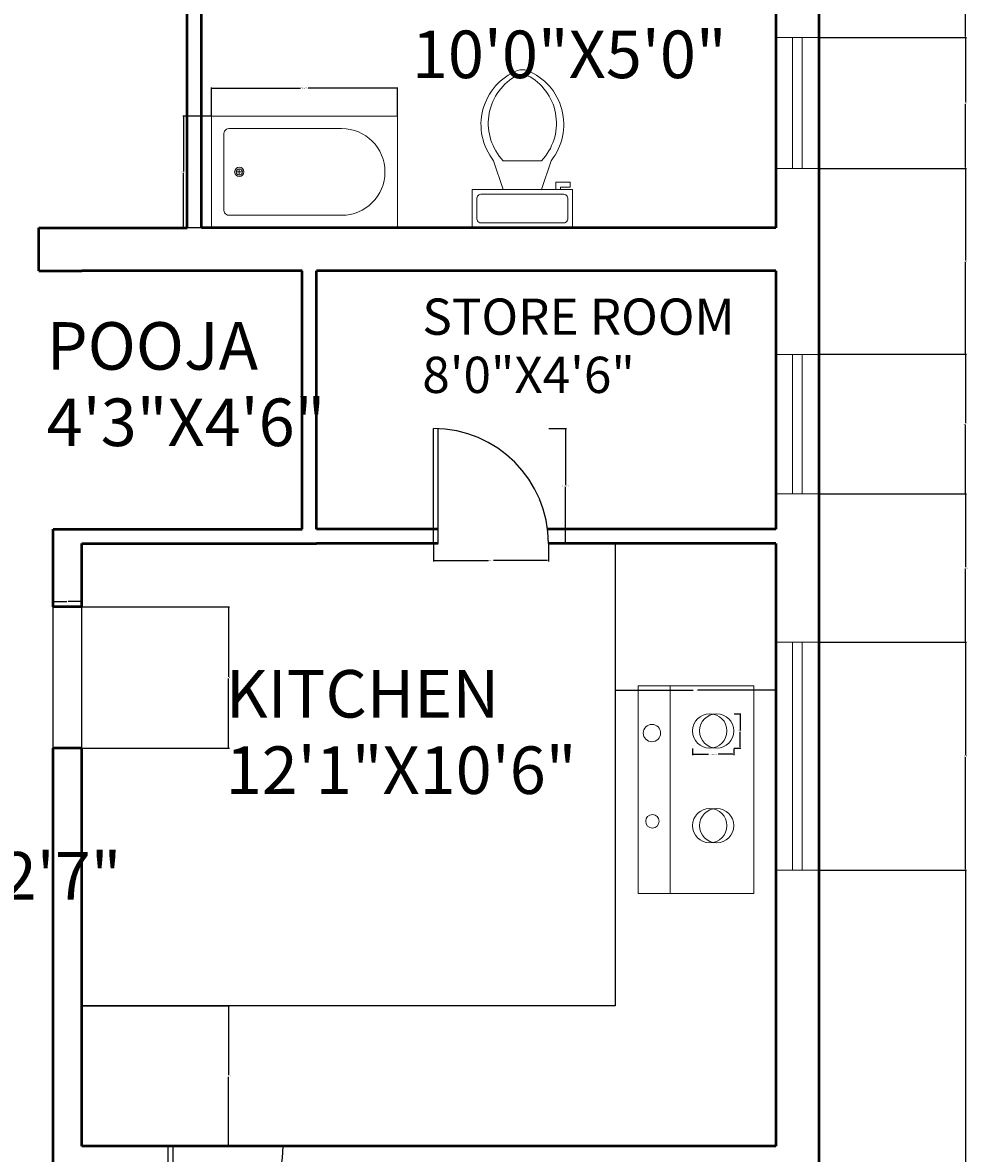
# Model space of a CAD drawing. Units: inches. Extents: x 614 to 1202, y 131 to 752.
# Tile 4 of 5: x 1005 to 1202, y 293 to 529. Entities that reach past the tile are written whole.
import ezdxf

# ---------------------------------------------------------------- set-up
doc = ezdxf.new("R2010")
doc.units = ezdxf.units.IN
doc.header["$MEASUREMENT"] = 0
for name, color, linetype, lineweight in [('A-ANNO-DIMS', 2, 'Continuous', 18), ('A-AREA-IDEN', 7, 'Continuous', 18), ('A-DOOR', 3, 'Continuous', 25), ('A-EQPM', 9, 'Continuous', 18), ('A-FLOR-CASE', 32, 'Continuous', 25), ('A-FLOR-FIXT', 9, 'Continuous', 18), ('A-GLAZ', 4, 'Continuous', 18), ('A-WALL', 7, 'Continuous', 50)]:
    doc.layers.add(name, color=color, linetype=linetype, lineweight=lineweight)
doc.styles.get("Standard").update_dxf_attribs({"font": 'arial.ttf'})
doc.dimstyles.get("Standard").update_dxf_attribs({"dimtxt": 0.18, "dimasz": 0.18, "dimexe": 0.18, "dimexo": 0.0625, "dimgap": 0.09, "dimtad": 0, "dimtih": 1, "dimtoh": 1, "dimdec": 0, "dimzin": 0, "dimdsep": 46, "dimlunit": 3, "dimtxsty": 'Standard', "dimcen": 0.09, "dimadec": 0, "dimazin": 0, "dimtfac": 1, "dimtdec": 0, "dimtofl": 0, "dimtmove": 0, "dimatfit": 3, "dimfxl": 1, "dimtolj": 1, "dimtzin": 0, "dimarcsym": 0})

# ---------------------------------------------------------------- blocks, each defined once
blk = doc.blocks.new('Bath Tub - 26 x 60 in.')
for p, q in [((8, -18), (10, -18)), ((9, -17), (9, -19))]:
    blk.add_line(p, q)
blk.add_lwpolyline([(0, -36), (0, 0), (60, 0), (60, -36)], close=True)
for points in [[(4, -30), (4, -6)], [(6, -4), (42, -4)], [(42, -32), (6, -32)]]:
    blk.add_lwpolyline(points)
for radius in [1.5, 1]:
    blk.add_circle((9, -18), radius)
for centre, radius, start, end in [((5.75, -5.75), 1.77, 81.8699, 188.1301), ((42, -18), 14, 270, 90), ((5.75, -30.25), 1.77, 171.8699, 278.1301)]:
    blk.add_arc(centre, radius, start, end)
blk = doc.blocks.new('Toilet - top')
for p, q in [((9.5, -6), (9.5, -2)), ((-10, -8.5), (-8, -8.5)), ((-10, -9.5), (-10, -8.5)), ((-8, -8.5), (-8, -8)), ((-7, -8), (-7, -9.5)), ((-4, -8), (-6, -14)), ((4, -8), (6, -14)), ((-7, -9.5), (-10, -9.5)), ((4, -14), (-4, -14))]:
    blk.add_line(p, q)
blk.add_lwpolyline([(10.5, -8), (10.5, 0), (-10.5, 0), (-10.5, -8)], close=True)
for points in [[(-9.5, -2), (-9.5, -6)], [(8.5, -1), (-8.5, -1)], [(-8.5, -7), (8.5, -7)]]:
    blk.add_lwpolyline(points)
for centre, radius, start, end in [((-8.62, -1.88), 0.884, 81.8699, 188.1301), ((8.62, -1.88), 0.884, 351.8699, 98.1301), ((-8.62, -6.12), 0.884, 171.8699, 278.1301), ((8.62, -6.12), 0.884, 261.8699, 8.1301), ((3.52, -21.58), 12.17, 141.4691, 247.9714), ((4.2, -21.82), 11.33, 136.3677, 238.9468), ((-3.52, -21.58), 12.17, 292.0284, 38.5307), ((-4.2, -21.82), 11.33, 301.053, 43.6321), ((0, -27.88), 4, 245.7318, 294.2682), ((0, -29), 4, 254.8605, 285.1395)]:
    blk.add_arc(centre, radius, start, end)
blk = doc.blocks.new('DOOR-SINGLE-24IN')
for p, q in [((0, 0), (0, 24)), ((1, 0), (1, 24))]:
    blk.add_line(p, q)
blk.add_arc((0, 0), 24, 0, 90)
blk = doc.blocks.new('COOKTOP-BURNER')
for centre in [(3.59, 3.59), (5.02, 3.59)]:
    blk.add_circle(centre, 3.59)
blk = doc.blocks.new('*D17')
at = {"layer": 'A-ANNO-DIMS', "color": 0, "lineweight": -2, "transparency": 16777216}
for p, q in [((1044.04, 509.64), (1044.04, 515.59)), ((1044.22, 515.41), (1062.66, 515.41)), ((1082.72, 515.41), (1064.29, 515.41)), ((1082.9, 509.64), (1082.9, 515.59))]:
    blk.add_line(p, q, dxfattribs=at)
at = {"layer": 'A-ANNO-DIMS', "color": 0, "transparency": 16777216}
for points in [[(1044.22, 515.44), (1044.22, 515.38), (1044.04, 515.41)], [(1082.72, 515.44), (1082.72, 515.38), (1082.9, 515.41)]]:
    blk.add_solid(points, dxfattribs=at)
at = {"layer": 'Defpoints', "color": 0, "transparency": 16777216}
for p in [(1082.9, 515.41), (1044.04, 509.58), (1082.9, 509.58)]:
    blk.add_point(p, dxfattribs=at)
at = {"layer": 'A-ANNO-DIMS', "color": 0, "transparency": 16777216, "insert": (1063.47, 515.41), "char_height": 0.18, "attachment_point": 5}
blk.add_mtext('\\A1;TUB 39 TYP.', dxfattribs=at)
blk = doc.blocks.new('*D18')
at = {"layer": 'A-ANNO-DIMS', "color": 0, "lineweight": -2, "transparency": 16777216}
for p, q in [((1043.98, 509.58), (1038.04, 509.58)), ((1038.22, 509.4), (1038.22, 498.1)), ((1038.22, 486.44), (1038.22, 497.74)), ((1043.98, 486.26), (1038.04, 486.26))]:
    blk.add_line(p, q, dxfattribs=at)
at = {"layer": 'A-ANNO-DIMS', "color": 0, "transparency": 16777216}
for points in [[(1038.19, 509.4), (1038.25, 509.4), (1038.22, 509.58)], [(1038.19, 486.44), (1038.25, 486.44), (1038.22, 486.26)]]:
    blk.add_solid(points, dxfattribs=at)
at = {"layer": 'Defpoints', "color": 0, "transparency": 16777216}
for p in [(1038.22, 509.58), (1044.04, 509.58), (1044.04, 486.26)]:
    blk.add_point(p, dxfattribs=at)
at = {"layer": 'A-ANNO-DIMS', "color": 0, "transparency": 16777216, "insert": (1038.22, 497.92), "char_height": 0.18, "attachment_point": 5}
blk.add_mtext('\\A1;23 TYP.', dxfattribs=at)
blk = doc.blocks.new('*D25')
at = {"layer": 'A-ANNO-DIMS', "color": 0, "lineweight": -2, "transparency": 16777216}
for p, q in [((1114.53, 444.26), (1118.24, 444.26)), ((1118.06, 444.08), (1118.06, 432.45)), ((1118.06, 420.44), (1118.06, 432.08)), ((1114.53, 420.26), (1118.24, 420.26))]:
    blk.add_line(p, q, dxfattribs=at)
at = {"layer": 'A-ANNO-DIMS', "color": 0, "transparency": 16777216}
for points in [[(1118.03, 444.08), (1118.09, 444.08), (1118.06, 444.26)], [(1118.03, 420.44), (1118.09, 420.44), (1118.06, 420.26)]]:
    blk.add_solid(points, dxfattribs=at)
at = {"layer": 'Defpoints', "color": 0, "transparency": 16777216}
for p in [(1114.46, 444.26), (1118.06, 444.26), (1114.46, 420.26)]:
    blk.add_point(p, dxfattribs=at)
at = {"layer": 'A-ANNO-DIMS', "color": 0, "transparency": 16777216, "insert": (1118.06, 432.26), "char_height": 0.18, "attachment_point": 5}
blk.add_mtext('\\A1;DOOR 24 TYP.', dxfattribs=at)
blk = doc.blocks.new('*D26')
at = {"layer": 'A-ANNO-DIMS', "color": 0, "lineweight": -2, "transparency": 16777216}
for p, q in [((1090.46, 420.2), (1090.46, 416.48)), ((1114.46, 420.2), (1114.46, 416.48)), ((1090.64, 416.66), (1101.94, 416.66)), ((1114.28, 416.66), (1102.99, 416.66))]:
    blk.add_line(p, q, dxfattribs=at)
at = {"layer": 'A-ANNO-DIMS', "color": 0, "transparency": 16777216}
for points in [[(1090.64, 416.69), (1090.64, 416.63), (1090.46, 416.66)], [(1114.28, 416.69), (1114.28, 416.63), (1114.46, 416.66)]]:
    blk.add_solid(points, dxfattribs=at)
at = {"layer": 'Defpoints', "color": 0, "transparency": 16777216}
for p in [(1090.46, 420.26), (1114.46, 420.26), (1114.46, 416.66)]:
    blk.add_point(p, dxfattribs=at)
at = {"layer": 'A-ANNO-DIMS', "color": 0, "transparency": 16777216, "insert": (1102.46, 416.66), "char_height": 0.18, "attachment_point": 5}
blk.add_mtext('\\A1;24 TYP.', dxfattribs=at)
blk = doc.blocks.new('*D29')
at = {"layer": 'A-ANNO-DIMS', "color": 0, "lineweight": -2, "transparency": 16777216}
for p, q in [((1144.6, 377.42), (1144.6, 376.01)), ((1144.78, 376.19), (1147.89, 376.19)), ((1153.04, 376.19), (1149.93, 376.19)), ((1153.22, 377.42), (1153.22, 376.01))]:
    blk.add_line(p, q, dxfattribs=at)
at = {"layer": 'A-ANNO-DIMS', "color": 0, "transparency": 16777216}
for points in [[(1144.78, 376.22), (1144.78, 376.16), (1144.6, 376.19)], [(1153.04, 376.22), (1153.04, 376.16), (1153.22, 376.19)]]:
    blk.add_solid(points, dxfattribs=at)
at = {"layer": 'Defpoints', "color": 0, "transparency": 16777216}
for p in [(1144.6, 377.48), (1153.22, 377.48), (1153.22, 376.19)]:
    blk.add_point(p, dxfattribs=at)
at = {"layer": 'A-ANNO-DIMS', "color": 0, "transparency": 16777216, "insert": (1148.91, 376.19), "char_height": 0.18, "attachment_point": 5}
blk.add_mtext('\\A1;BURNER 9 TYP.', dxfattribs=at)
blk = doc.blocks.new('*D30')
at = {"layer": 'A-ANNO-DIMS', "color": 0, "lineweight": -2, "transparency": 16777216}
for p, q in [((1153.28, 384.66), (1154.69, 384.66)), ((1154.51, 384.48), (1154.51, 381.25)), ((1154.51, 377.66), (1154.51, 380.89)), ((1153.28, 377.48), (1154.69, 377.48))]:
    blk.add_line(p, q, dxfattribs=at)
at = {"layer": 'A-ANNO-DIMS', "color": 0, "transparency": 16777216}
for points in [[(1154.48, 384.48), (1154.54, 384.48), (1154.51, 384.66)], [(1154.48, 377.66), (1154.54, 377.66), (1154.51, 377.48)]]:
    blk.add_solid(points, dxfattribs=at)
at = {"layer": 'Defpoints', "color": 0, "transparency": 16777216}
for p in [(1153.22, 384.66), (1154.51, 384.66), (1153.22, 377.48)]:
    blk.add_point(p, dxfattribs=at)
at = {"layer": 'A-ANNO-DIMS', "color": 0, "transparency": 16777216, "insert": (1154.51, 381.07), "char_height": 0.18, "attachment_point": 5}
blk.add_mtext('\\A1;7 TYP.', dxfattribs=at)
blk = doc.blocks.new('*D54')
at = {"layer": 'A-ANNO-DIMS', "color": 0, "lineweight": -2, "transparency": 16777216}
for p, q in [((1171.06, 595), (1201.82, 595)), ((1201.64, 594.82), (1201.64, 560.69)), ((1201.64, 526.2), (1201.64, 560.33)), ((1171.06, 526.02), (1201.82, 526.02))]:
    blk.add_line(p, q, dxfattribs=at)
at = {"layer": 'A-ANNO-DIMS', "color": 0, "transparency": 16777216}
for points in [[(1201.61, 594.82), (1201.67, 594.82), (1201.64, 595)], [(1201.61, 526.2), (1201.67, 526.2), (1201.64, 526.02)]]:
    blk.add_solid(points, dxfattribs=at)
at = {"layer": 'Defpoints', "color": 0, "transparency": 16777216}
for p in [(1170.99, 595), (1201.64, 595), (1170.99, 526.02)]:
    blk.add_point(p, dxfattribs=at)
at = {"layer": 'A-ANNO-DIMS', "color": 0, "transparency": 16777216, "insert": (1201.64, 560.51), "char_height": 0.18, "attachment_point": 5}
blk.add_mtext('\\A1;68.99', dxfattribs=at)
blk = doc.blocks.new('*D55')
at = {"layer": 'A-ANNO-DIMS', "color": 0, "lineweight": -2, "transparency": 16777216}
for p, q in [((1171.06, 526.02), (1201.82, 526.02)), ((1201.64, 525.84), (1201.64, 512.51)), ((1201.64, 498.81), (1201.64, 512.14)), ((1171.06, 498.63), (1201.82, 498.63))]:
    blk.add_line(p, q, dxfattribs=at)
at = {"layer": 'A-ANNO-DIMS', "color": 0, "transparency": 16777216}
for points in [[(1201.61, 525.84), (1201.67, 525.84), (1201.64, 526.02)], [(1201.61, 498.81), (1201.67, 498.81), (1201.64, 498.63)]]:
    blk.add_solid(points, dxfattribs=at)
at = {"layer": 'Defpoints', "color": 0, "transparency": 16777216}
for p in [(1170.99, 526.02), (1201.64, 526.02), (1170.99, 498.63)]:
    blk.add_point(p, dxfattribs=at)
at = {"layer": 'A-ANNO-DIMS', "color": 0, "transparency": 16777216, "insert": (1201.64, 512.32), "char_height": 0.18, "attachment_point": 5}
blk.add_mtext('\\A1;27.38', dxfattribs=at)
blk = doc.blocks.new('*D56')
at = {"layer": 'A-ANNO-DIMS', "color": 0, "lineweight": -2, "transparency": 16777216}
for p, q in [((1171.06, 498.63), (1201.82, 498.63)), ((1201.64, 498.45), (1201.64, 479.39)), ((1201.64, 459.97), (1201.64, 479.03)), ((1171.06, 459.79), (1201.82, 459.79))]:
    blk.add_line(p, q, dxfattribs=at)
at = {"layer": 'A-ANNO-DIMS', "color": 0, "transparency": 16777216}
for points in [[(1201.61, 498.45), (1201.67, 498.45), (1201.64, 498.63)], [(1201.61, 459.97), (1201.67, 459.97), (1201.64, 459.79)]]:
    blk.add_solid(points, dxfattribs=at)
at = {"layer": 'Defpoints', "color": 0, "transparency": 16777216}
for p in [(1170.99, 498.63), (1201.64, 498.63), (1170.99, 459.79)]:
    blk.add_point(p, dxfattribs=at)
at = {"layer": 'A-ANNO-DIMS', "color": 0, "transparency": 16777216, "insert": (1201.64, 479.21), "char_height": 0.18, "attachment_point": 5}
blk.add_mtext('\\A1;38.85', dxfattribs=at)
blk = doc.blocks.new('*D57')
at = {"layer": 'A-ANNO-DIMS', "color": 0, "lineweight": -2, "transparency": 16777216}
for p, q in [((1171.06, 459.79), (1201.82, 459.79)), ((1201.64, 459.61), (1201.64, 445.38)), ((1201.64, 430.79), (1201.64, 445.02)), ((1171.06, 430.61), (1201.82, 430.61))]:
    blk.add_line(p, q, dxfattribs=at)
at = {"layer": 'A-ANNO-DIMS', "color": 0, "transparency": 16777216}
for points in [[(1201.61, 459.61), (1201.67, 459.61), (1201.64, 459.79)], [(1201.61, 430.79), (1201.67, 430.79), (1201.64, 430.61)]]:
    blk.add_solid(points, dxfattribs=at)
at = {"layer": 'Defpoints', "color": 0, "transparency": 16777216}
for p in [(1170.99, 459.79), (1201.64, 459.79), (1170.99, 430.61)]:
    blk.add_point(p, dxfattribs=at)
at = {"layer": 'A-ANNO-DIMS', "color": 0, "transparency": 16777216, "insert": (1201.64, 445.2), "char_height": 0.18, "attachment_point": 5}
blk.add_mtext('\\A1;29.177', dxfattribs=at)
blk = doc.blocks.new('*D58')
at = {"layer": 'A-ANNO-DIMS', "color": 0, "lineweight": -2, "transparency": 16777216}
for p, q in [((1171.06, 430.61), (1201.82, 430.61)), ((1201.64, 430.43), (1201.64, 415.29)), ((1201.64, 399.79), (1201.64, 414.93)), ((1171.06, 399.61), (1201.82, 399.61))]:
    blk.add_line(p, q, dxfattribs=at)
at = {"layer": 'A-ANNO-DIMS', "color": 0, "transparency": 16777216}
for points in [[(1201.61, 430.43), (1201.67, 430.43), (1201.64, 430.61)], [(1201.61, 399.79), (1201.67, 399.79), (1201.64, 399.61)]]:
    blk.add_solid(points, dxfattribs=at)
at = {"layer": 'Defpoints', "color": 0, "transparency": 16777216}
for p in [(1170.99, 430.61), (1201.64, 430.61), (1170.99, 399.61)]:
    blk.add_point(p, dxfattribs=at)
at = {"layer": 'A-ANNO-DIMS', "color": 0, "transparency": 16777216, "insert": (1201.64, 415.11), "char_height": 0.18, "attachment_point": 5}
blk.add_mtext('\\A1;31.004', dxfattribs=at)
blk = doc.blocks.new('*D59')
at = {"layer": 'A-ANNO-DIMS', "color": 0, "lineweight": -2, "transparency": 16777216}
for p, q in [((1171.06, 399.61), (1201.82, 399.61)), ((1201.64, 399.43), (1201.64, 375.97)), ((1201.64, 352.15), (1201.64, 375.61)), ((1171.06, 351.97), (1201.82, 351.97))]:
    blk.add_line(p, q, dxfattribs=at)
at = {"layer": 'A-ANNO-DIMS', "color": 0, "transparency": 16777216}
for points in [[(1201.61, 399.43), (1201.67, 399.43), (1201.64, 399.61)], [(1201.61, 352.15), (1201.67, 352.15), (1201.64, 351.97)]]:
    blk.add_solid(points, dxfattribs=at)
at = {"layer": 'Defpoints', "color": 0, "transparency": 16777216}
for p in [(1170.99, 399.61), (1201.64, 399.61), (1170.99, 351.97)]:
    blk.add_point(p, dxfattribs=at)
at = {"layer": 'A-ANNO-DIMS', "color": 0, "transparency": 16777216, "insert": (1201.64, 375.79), "char_height": 0.18, "attachment_point": 5}
blk.add_mtext('\\A1;47.63', dxfattribs=at)
blk = doc.blocks.new('*D60')
at = {"layer": 'A-ANNO-DIMS', "color": 0, "lineweight": -2, "transparency": 16777216}
for p, q in [((1171.06, 351.97), (1201.82, 351.97)), ((1201.64, 351.79), (1201.64, 287.3)), ((1201.64, 222.44), (1201.64, 286.94)), ((1171.06, 222.26), (1201.82, 222.26))]:
    blk.add_line(p, q, dxfattribs=at)
at = {"layer": 'A-ANNO-DIMS', "color": 0, "transparency": 16777216}
for points in [[(1201.61, 351.79), (1201.67, 351.79), (1201.64, 351.97)], [(1201.61, 222.44), (1201.67, 222.44), (1201.64, 222.26)]]:
    blk.add_solid(points, dxfattribs=at)
at = {"layer": 'Defpoints', "color": 0, "transparency": 16777216}
for p in [(1170.99, 351.97), (1201.64, 351.97), (1170.99, 222.26)]:
    blk.add_point(p, dxfattribs=at)
at = {"layer": 'A-ANNO-DIMS', "color": 0, "transparency": 16777216, "insert": (1201.64, 287.12), "char_height": 0.18, "attachment_point": 5}
blk.add_mtext('\\A1;129.7', dxfattribs=at)
blk = doc.blocks.new('*D71')
at = {"layer": 'A-ANNO-DIMS', "color": 0, "lineweight": -2, "transparency": 16777216}
for p, q in [((1010.99, 377.51), (1010.99, 408.28)), ((1011.17, 408.1), (1013.84, 408.1)), ((1016.81, 408.1), (1014.14, 408.1)), ((1016.99, 377.51), (1016.99, 408.28))]:
    blk.add_line(p, q, dxfattribs=at)
at = {"layer": 'A-ANNO-DIMS', "color": 0, "transparency": 16777216}
for points in [[(1011.17, 408.13), (1011.17, 408.07), (1010.99, 408.1)], [(1016.81, 408.13), (1016.81, 408.07), (1016.99, 408.1)]]:
    blk.add_solid(points, dxfattribs=at)
at = {"layer": 'Defpoints', "color": 0, "transparency": 16777216}
for p in [(1016.99, 408.1), (1010.99, 377.45), (1016.99, 377.45)]:
    blk.add_point(p, dxfattribs=at)
at = {"layer": 'A-ANNO-DIMS', "color": 0, "transparency": 16777216, "insert": (1013.99, 408.1), "char_height": 0.18, "attachment_point": 5}
blk.add_mtext('\\A1;6', dxfattribs=at)
blk = doc.blocks.new('*D76')
at = {"layer": 'A-ANNO-DIMS', "color": 0, "lineweight": -2, "transparency": 16777216}
for p, q in [((1017.06, 323.63), (1047.82, 323.63)), ((1047.64, 323.45), (1047.64, 309.13)), ((1047.64, 294.44), (1047.64, 308.76)), ((1017.06, 294.26), (1047.82, 294.26))]:
    blk.add_line(p, q, dxfattribs=at)
at = {"layer": 'A-ANNO-DIMS', "color": 0, "transparency": 16777216}
for points in [[(1047.61, 323.45), (1047.67, 323.45), (1047.64, 323.63)], [(1047.61, 294.44), (1047.67, 294.44), (1047.64, 294.26)]]:
    blk.add_solid(points, dxfattribs=at)
at = {"layer": 'Defpoints', "color": 0, "transparency": 16777216}
for p in [(1016.99, 323.63), (1016.99, 294.26), (1047.64, 294.26)]:
    blk.add_point(p, dxfattribs=at)
at = {"layer": 'A-ANNO-DIMS', "color": 0, "transparency": 16777216, "insert": (1047.64, 308.95), "char_height": 0.18, "attachment_point": 5}
blk.add_mtext('\\A1;29.364', dxfattribs=at)
blk = doc.blocks.new('*D77')
at = {"layer": 'A-ANNO-DIMS', "color": 0, "lineweight": -2, "transparency": 16777216}
for p, q in [((1128.44, 420.2), (1128.44, 389.43)), ((1161.99, 420.2), (1161.99, 389.43)), ((1128.62, 389.61), (1144.75, 389.61)), ((1161.81, 389.61), (1145.68, 389.61))]:
    blk.add_line(p, q, dxfattribs=at)
at = {"layer": 'A-ANNO-DIMS', "color": 0, "transparency": 16777216}
for points in [[(1128.62, 389.64), (1128.62, 389.58), (1128.44, 389.61)], [(1161.81, 389.64), (1161.81, 389.58), (1161.99, 389.61)]]:
    blk.add_solid(points, dxfattribs=at)
at = {"layer": 'Defpoints', "color": 0, "transparency": 16777216}
for p in [(1128.44, 420.26), (1161.99, 420.26), (1128.44, 389.61)]:
    blk.add_point(p, dxfattribs=at)
at = {"layer": 'A-ANNO-DIMS', "color": 0, "transparency": 16777216, "insert": (1145.22, 389.61), "char_height": 0.18, "attachment_point": 5}
blk.add_mtext('\\A1;33.554', dxfattribs=at)
blk = doc.blocks.new('*D78')
at = {"layer": 'A-ANNO-DIMS', "color": 0, "lineweight": -2, "transparency": 16777216}
for p, q in [((1017.06, 406.99), (1047.82, 406.99)), ((1047.64, 406.81), (1047.64, 392.4)), ((1047.64, 377.63), (1047.64, 392.04)), ((1017.06, 377.45), (1047.82, 377.45))]:
    blk.add_line(p, q, dxfattribs=at)
at = {"layer": 'A-ANNO-DIMS', "color": 0, "transparency": 16777216}
for points in [[(1047.61, 406.81), (1047.67, 406.81), (1047.64, 406.99)], [(1047.61, 377.63), (1047.67, 377.63), (1047.64, 377.45)]]:
    blk.add_solid(points, dxfattribs=at)
at = {"layer": 'Defpoints', "color": 0, "transparency": 16777216}
for p in [(1016.99, 406.99), (1016.99, 377.45), (1047.64, 377.45)]:
    blk.add_point(p, dxfattribs=at)
at = {"layer": 'A-ANNO-DIMS', "color": 0, "transparency": 16777216, "insert": (1047.64, 392.22), "char_height": 0.18, "attachment_point": 5}
blk.add_mtext('\\A1;29.54', dxfattribs=at)

msp = doc.modelspace()

# ---------------------------------------------------------------- linework, layer by layer
at = {"layer": 'A-DOOR'}
for p, q in [((1090.4646, 420.2636), (1091.4646, 420.2636)), ((1034.9545, 294.2636), (1058.9545, 294.2636))]:
    msp.add_line(p, q, dxfattribs=at)
at = {"layer": 'A-EQPM'}
msp.add_line((1139.9384, 390.4763), (1139.9384, 347.0703), dxfattribs=at)
msp.add_lwpolyline([(1133.1941, 390.4763), (1157.3823, 390.4763), (1157.3823, 347.0703), (1133.1941, 347.0703)], close=True, dxfattribs=at)
for centre, radius in [((1136.1044, 380.6252), 1.814), ((1136.2053, 362.1833), 1.4109)]:
    msp.add_circle(centre, radius, dxfattribs=at)
at = {"layer": 'A-FLOR-CASE'}
for p, q in [((1128.4399, 420.2636), (1128.4399, 323.6273)), ((1128.4399, 323.6273), (1016.9938, 323.6273))]:
    msp.add_line(p, q, dxfattribs=at)
at = {"layer": 'A-GLAZ'}
for p, q in [((1170.9938, 526.0154), (1161.9938, 526.0154)), ((1165.4938, 498.634), (1165.4938, 526.0154)), ((1166.4938, 526.0154), (1170.9938, 526.0154)), ((1167.4938, 498.634), (1167.4938, 526.0154)), ((1161.9938, 498.634), (1170.9938, 498.634)), ((1170.9938, 459.7869), (1161.9938, 459.7869)), ((1165.4938, 430.6102), (1165.4938, 459.7869)), ((1166.4938, 459.7869), (1170.9938, 459.7869)), ((1167.4938, 430.6102), (1167.4938, 459.7869)), ((1161.9938, 430.6102), (1170.9938, 430.6102)), ((1161.9938, 399.6057), (1170.9938, 399.6057)), ((1165.4938, 399.6057), (1165.4938, 351.971)), ((1167.4938, 399.6057), (1167.4938, 351.971)), ((1166.4938, 351.971), (1161.9938, 351.971)), ((1161.9938, 351.971), (1170.9938, 351.971))]:
    msp.add_line(p, q, dxfattribs=at)
at = {"layer": 'A-WALL'}
for p, q in [((1170.9938, 721.2636), (1170.9938, 222.2636)), ((1038.9938, 486.2636), (1038.9938, 546.2636)), ((1041.9938, 486.2636), (1041.9938, 546.2636)), ((1161.9938, 546.2636), (1161.9938, 486.2636)), ((1170.9938, 546.2636), (1170.9938, 486.2636)), ((1007.9938, 477.2636), (1007.9938, 486.2636)), ((1007.9938, 486.2636), (1016.9938, 486.2636)), ((1016.9938, 486.2636), (1038.9938, 486.2636)), ((1161.9938, 486.2636), (1041.9938, 486.2636)), ((1007.9938, 477.2636), (1016.9938, 477.2636)), ((1062.9938, 477.2636), (1016.9938, 477.2636)), ((1062.9938, 423.2636), (1062.9938, 477.2636)), ((1161.9938, 477.2636), (1065.9938, 477.2636)), ((1065.9938, 423.2636), (1065.9938, 477.2636)), ((1161.9938, 477.2636), (1161.9938, 423.2636)), ((1170.9938, 477.2636), (1170.9938, 423.2636)), ((1010.9938, 423.2636), (1062.9938, 423.2636)), ((1010.9938, 406.9916), (1010.9938, 423.2636)), ((1091.4646, 423.2636), (1065.9938, 423.2636)), ((1161.9938, 423.2636), (1114.2764, 423.2636)), ((1016.9938, 420.2636), (1065.9938, 420.2636)), ((1016.9938, 406.9916), (1016.9938, 420.2636)), ((1091.4646, 420.2636), (1065.9938, 420.2636)), ((1161.9938, 420.2636), (1114.4646, 420.2636)), ((1161.9938, 420.2636), (1161.9938, 294.2636)), ((1016.9938, 406.9916), (1010.9938, 406.9916)), ((1010.9938, 294.2636), (1010.9938, 377.4494)), ((1010.9938, 255.2636), (1010.9938, 377.4494)), ((1010.9938, 264.2636), (1010.9938, 377.4494)), ((1016.9938, 377.4494), (1010.9938, 377.4494)), ((1016.9938, 294.2636), (1016.9938, 377.4494)), ((1161.9938, 294.2636), (1016.9938, 294.2636))]:
    msp.add_line(p, q, dxfattribs=at)

# ---------------------------------------------------------------- block references
at = {"layer": 'A-DOOR'}
msp.add_blockref('DOOR-SINGLE-24IN', (1090.465, 420.264), dxfattribs=at)
at = {"layer": 'A-DOOR', "extrusion": (0, 0, -1), "zscale": -1, "rotation": 180}
msp.add_blockref('DOOR-SINGLE-24IN', (-1034.9549, 294.2632), dxfattribs=at)
at = {"layer": 'A-EQPM'}
for p in [(1144.602, 377.479), (1144.602, 357.6841)]:
    msp.add_blockref('COOKTOP-BURNER', p, dxfattribs=at)
at = {"layer": 'A-FLOR-FIXT', "rotation": 180}
msp.add_blockref('Toilet - top', (1109.0245, 486.2636), dxfattribs=at)
at = {"layer": 'A-FLOR-FIXT', "xscale": 0.6476301684216574, "yscale": 0.6476301684216574, "zscale": 0.6476301684216574}
msp.add_blockref('Bath Tub - 26 x 60 in.', (1044.0441, 509.5783), dxfattribs=at)

# ---------------------------------------------------------------- texts
at = {"layer": 'A-AREA-IDEN'}
for s, height, p in [('10\'0"X5\'0"', 9.93672, (1085.9373, 517.523)), ('STORE ROOM', 7.57382, (1088.123, 463.8785)), ('POOJA ', 9.93672, (1009.6138, 456.5773)), ('8\'0"X4\'6"', 7.57382, (1088.123, 451.7119)), ('4\'3"X4\'6"', 9.93672, (1009.6138, 440.6148)), ('KITCHEN ', 9.93672, (1047.036, 383.8579)), ('12\'1"X10\'6"', 9.93672, (1047.036, 367.8954)), ('12\'0"X12\'7"', 9.93672, (951.9517, 345.8279))]:
    msp.add_text(s, height=height, dxfattribs=at).set_placement(p)

# ---------------------------------------------------------------- dimensions: what is measured, and where the dimension line sits
at = {"layer": 'A-ANNO-DIMS'}
for base, p1, p2, angle, override, picture, middle in [((1201.6438, 595.0017), (1170.9938, 526.0154), (1170.9938, 595.0017), 90, {"dimdec": 2, "dimlfac": 1, "dimrnd": 0, "dimzin": 0, "dimdsep": 46, "dimlunit": 2}, '*D54', (1201.6438, 560.5085)), ((1201.6438, 526.0154), (1170.9938, 498.634), (1170.9938, 526.0154), 90, {"dimdec": 2, "dimlfac": 1, "dimrnd": 0, "dimzin": 0, "dimdsep": 46, "dimlunit": 2}, '*D55', (1201.6438, 512.3247)), ((1201.6438, 498.634), (1170.9938, 459.7869), (1170.9938, 498.634), 90, {"dimdec": 2, "dimlfac": 1, "dimrnd": 0, "dimzin": 0, "dimdsep": 46, "dimlunit": 2}, '*D56', (1201.6438, 479.2105)), ((1201.6438, 459.7869), (1170.9938, 430.6102), (1170.9938, 459.7869), 90, {"dimdec": 3, "dimlfac": 1, "dimrnd": 0, "dimzin": 0, "dimdsep": 46, "dimlunit": 2}, '*D57', (1201.6438, 445.1985)), ((1201.64376, 430.61015), (1170.99376, 399.6057), (1170.99376, 430.61015), 90, {"dimdec": 3, "dimlfac": 1, "dimrnd": 0, "dimzin": 0, "dimdsep": 46, "dimlunit": 2}, '*D58', (1201.64376, 415.10792)), ((1128.4399, 389.6136), (1161.9938, 420.2636), (1128.4399, 420.2636), 180, {"dimdec": 3, "dimlfac": 1, "dimrnd": 0, "dimzin": 0, "dimdsep": 46, "dimlunit": 2}, '*D77', (1145.2168, 389.6136)), ((1047.6438, 377.4494), (1016.9938, 406.9916), (1016.9938, 377.4494), 270, {"dimdec": 2, "dimlfac": 1, "dimrnd": 0, "dimzin": 0, "dimdsep": 46, "dimlunit": 2}, '*D78', (1047.6438, 392.2205)), ((1201.6438, 399.6057), (1170.9938, 351.971), (1170.9938, 399.6057), 90, {"dimdec": 2, "dimlfac": 1, "dimrnd": 0, "dimzin": 0, "dimdsep": 46, "dimlunit": 2}, '*D59', (1201.6438, 375.7884)), ((1201.6438, 351.971), (1170.9938, 222.2636), (1170.9938, 351.971), 90, {"dimdec": 1, "dimlfac": 1, "dimrnd": 0, "dimzin": 0, "dimdsep": 46, "dimlunit": 2}, '*D60', (1201.6438, 287.1173)), ((1047.6438, 294.2636), (1016.9938, 323.6273), (1016.9938, 294.2636), 270, {"dimdec": 3, "dimlfac": 1, "dimrnd": 0, "dimzin": 0, "dimdsep": 46, "dimlunit": 2}, '*D76', (1047.6438, 308.9454))]:
    dim = msp.add_linear_dim(base=base, p1=p1, p2=p2, angle=angle, dimstyle='Standard', override=override, dxfattribs=at)
    dim.commit()
    dim.dimension.update_dxf_attribs({"geometry": picture, "text_midpoint": middle})
for base, p1, p2, text, picture, middle in [((1082.9019, 515.4069), (1044.0441, 509.5783), (1082.9019, 509.5783), 'TUB <> TYP.', '*D17', (1063.473, 515.4069)), ((1114.4646, 416.6636), (1090.4646, 420.2636), (1114.4646, 420.2636), '<> TYP.', '*D26', (1102.4646, 416.6636)), ((1153.2167, 376.1864), (1144.602, 377.4787), (1153.2167, 377.4787), 'BURNER <> TYP.', '*D29', (1148.9093, 376.1864))]:
    dim = msp.add_linear_dim(base=base, p1=p1, p2=p2, text=text, dimstyle='Standard', override={"dimdec": 0, "dimlfac": 1, "dimrnd": 0, "dimzin": 0, "dimdsep": 46, "dimlunit": 2}, dxfattribs=at)
    dim.commit()
    dim.dimension.update_dxf_attribs({"geometry": picture, "text_midpoint": middle})
for base, p1, p2, text, picture, middle in [((1038.2154, 509.5783), (1044.0441, 486.2636), (1044.0441, 509.5783), '<> TYP.', '*D18', (1038.2154, 497.9209)), ((1118.0646, 444.2636), (1114.4646, 420.2636), (1114.4646, 444.2636), 'DOOR <> TYP.', '*D25', (1118.0646, 432.2636)), ((1154.5089, 384.6638), (1153.2167, 377.4787), (1153.2167, 384.6638), '<> TYP.', '*D30', (1154.5089, 381.0712))]:
    dim = msp.add_linear_dim(base=base, p1=p1, p2=p2, angle=90, text=text, dimstyle='Standard', override={"dimdec": 0, "dimlfac": 1, "dimrnd": 0, "dimzin": 0, "dimdsep": 46, "dimlunit": 2}, dxfattribs=at)
    dim.commit()
    dim.dimension.update_dxf_attribs({"geometry": picture, "text_midpoint": middle})
dim = msp.add_linear_dim(base=(1016.9938, 408.0994), p1=(1010.9938, 377.4494), p2=(1016.9938, 377.4494), dimstyle='Standard', override={"dimdec": 0, "dimlfac": 1, "dimrnd": 0, "dimzin": 0, "dimdsep": 46, "dimlunit": 2}, dxfattribs=at)
dim.commit()
dim.dimension.update_dxf_attribs({"geometry": '*D71', "text_midpoint": (1013.9938, 408.0994)})

doc.saveas('drawing.dxf')
